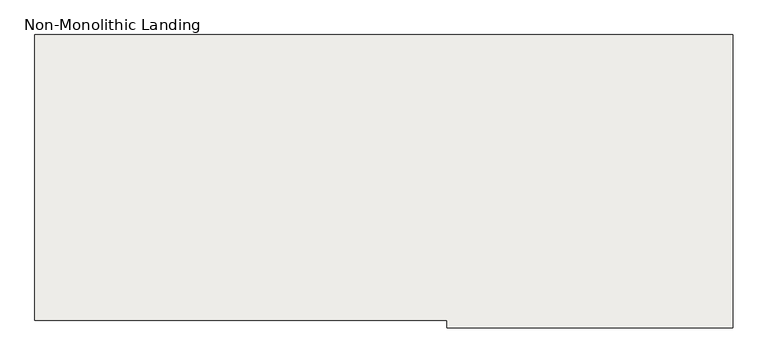
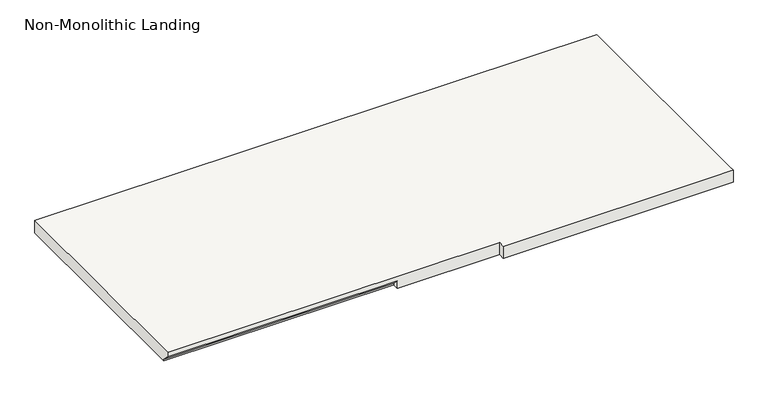
"""IFC4 building model written with IfcOpenShell, lengths in millimetres: slab geometry, Non-Monolithic Landing."""

from ifc_helpers import new_model, si_unit, origin, place, context, project, spatial, faceted_brep, source, transform, mapped, element, save


def non_monolithic_landing_2d4b1833(model_context):
    return source(origin(), model_context, "Body", "Brep", [
        faceted_brep([(-3617.4415084, -19522.1851539, 33682.2339133), (-3617.4415084, -19496.7851539, 33656.8339133), (-2703.0415084, -19496.7851539, 33656.8339133), (-2703.0415084, -19522.1851539, 33682.2339133), (-2296.6415084, -19522.1851539, 33701.2839133), (-2296.6415084, -19547.5851539, 33701.2839133), (-1382.2415084, -19547.5851539, 33701.2839133), (-1382.2415084, -19522.1851539, 33701.2839133), (-1382.2415084, -18607.7851539, 33701.2839133), (-3617.4415084, -18607.7851539, 33701.2839133), (-3617.4415084, -19522.1851539, 33701.2839133), (-2703.0415084, -19496.7851539, 33650.4839133), (-3617.4415084, -19496.7851539, 33650.4839133), (-3617.4415084, -18607.7851539, 33650.4839133), (-1382.2415084, -18607.7851539, 33650.4839133), (-1382.2415084, -19522.1851539, 33650.4839133), (-1382.2415084, -19547.5851539, 33650.4839133), (-2296.6415084, -19547.5851539, 33650.4839133), (-2296.6415084, -19522.1851539, 33650.4839133), (-2703.0415084, -19522.1851539, 33650.4839133)], [[[0, 1, 2, 3]], [[4, 5, 6, 7, 8, 9, 10]], [[11, 12, 13, 14, 15, 16, 17, 18, 19]], [[12, 11, 2, 1]], [[11, 19, 3, 2]], [[4, 10, 0, 3, 19, 18]], [[5, 4, 18, 17]], [[6, 5, 17, 16]], [[7, 6, 16, 15]], [[8, 7, 15, 14]], [[9, 8, 14, 13]], [[10, 9, 13, 12, 1, 0]]]),
    ])


if __name__ == "__main__":
    model = new_model("IFC4")
    model_context = context("Model", 3, world=origin())
    ifc_project = project(units=[si_unit("LENGTHUNIT", "METRE", prefix="MILLI")], contexts=[model_context])
    site = spatial("IfcSite", under=ifc_project)
    building = spatial("IfcBuilding", under=site)
    placement = place(None, origin())
    non_monolithic_landing_shape = non_monolithic_landing_2d4b1833(model_context)
    element("IfcSlab", 1, ObjectType="Non-Monolithic Landing", at=placement, inside=building, context=model_context, shape_type="MappedRepresentation", body=[
        mapped(non_monolithic_landing_shape, transform((0.0, 0.0, 0.0), x_axis=(1.0, 0.0, 0.0), y_axis=(0.0, 1.0, 0.0), z_axis=(0.0, 0.0, 1.0))),
    ])
    save(model, "model.ifc")
